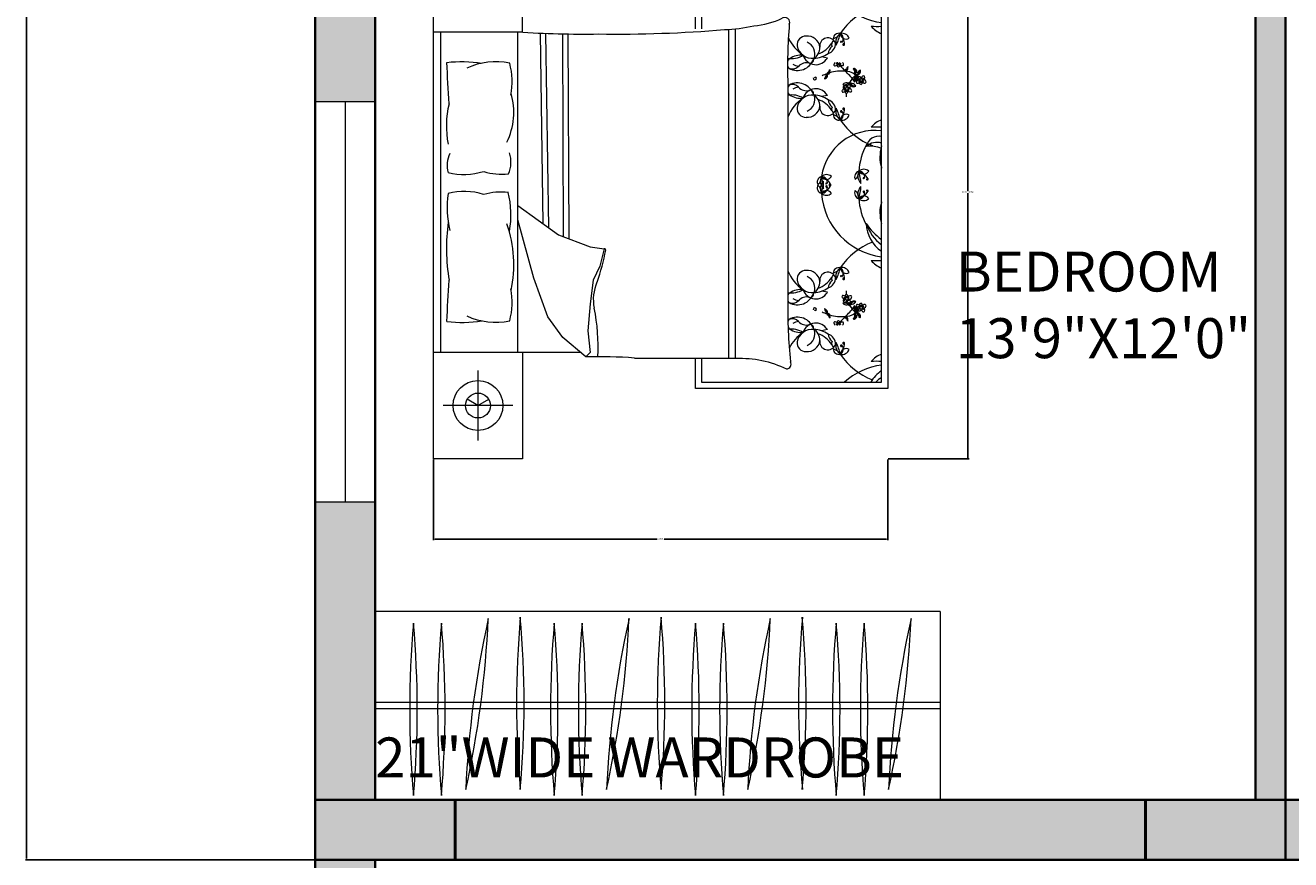
# Model space of a CAD drawing. Units: inches. Extents: x -28 to 485, y -861 to 54.
# Tile 6 of 14: x -28 to 162, y -365 to -240. Entities that reach past the tile are written whole.
import ezdxf

# ---------------------------------------------------------------- set-up
doc = ezdxf.new("R2010")
doc.units = ezdxf.units.IN
doc.header["$MEASUREMENT"] = 0
for name, color, linetype, lineweight in [('A-ANNO-DIMS', 2, 'Continuous', 18), ('A-ANNO-TEXT', 7, 'Continuous', 18), ('A-AREA-IDEN', 7, 'Continuous', 18), ('A-COLS', 7, 'Continuous', 50), ('A-COLS-PATT', 8, 'Continuous', 13), ('A-FLOR-CASE', 8, 'Continuous', 18), ('A-FURN', 8, 'Continuous', 13), ('A-GLAZ', 4, 'Continuous', 18), ('A-WALL', 7, 'Continuous', 35), ('A-WALL-PATT', 34, 'Continuous', 13)]:
    doc.layers.add(name, color=color, linetype=linetype, lineweight=lineweight)
doc.styles.get("Standard").update_dxf_attribs({"font": 'arial.ttf'})
doc.dimstyles.get("Standard").update_dxf_attribs({"dimtxt": 0.18, "dimasz": 0.18, "dimexe": 0.18, "dimexo": 0.0625, "dimgap": 0.09, "dimtad": 0, "dimtih": 1, "dimtoh": 1, "dimdec": 0, "dimzin": 0, "dimdsep": 46, "dimlunit": 3, "dimtxsty": 'Standard', "dimcen": 0.09, "dimadec": 0, "dimazin": 0, "dimtfac": 1, "dimtdec": 0, "dimtofl": 0, "dimtmove": 0, "dimatfit": 3, "dimfxl": 1, "dimtolj": 1, "dimtzin": 0, "dimarcsym": 0})

# ---------------------------------------------------------------- blocks, each defined once
blk = doc.blocks.new('BED-DOUBLE-WITH-NIGHTSTANDS')
for p, q in [((0, 0), (0, 80.08)), ((6.67, 66.84), (6.67, 77.31)), ((11.91, 72.08), (1.44, 72.08)), ((39.26, 64.51), (39.26, 68.96)), ((39.26, 68.96), (68.11, 68.96)), ((68.11, 68.96), (68.11, 10.57)), ((40.19, 68.03), (40.19, 64.5)), ((67.18, 68.03), (40.19, 68.03)), ((67.18, 11.5), (67.18, 68.03)), ((45.25, 64.51), (45.25, 15.09)), ((1.03, 64.07), (1.03, 16.02)), ((12.66, 16.02), (12.66, 64.07)), ((15.98, 63.85), (16.38, 35.34)), ((16.8, 63.82), (17.22, 34.74)), ((19.33, 63.78), (19.45, 33.37)), ((20.15, 63.78), (20.27, 33.06)), ((44.25, 64.43), (44.25, 15.09)), ((59.06, 60.14), (58.15, 60.31)), ((53.12, 56.3), (53.12, 23.78)), ((59.06, 54.54), (58.15, 54.36)), ((12.66, 38.02), (18.76, 33.63)), ((15.04, 27.14), (12.66, 35.87)), ((18.76, 33.63), (23.47, 31.84)), ((23.47, 31.84), (25.57, 31.52)), ((25.57, 31.52), (24.92, 28.93)), ((24.92, 28.93), (23.95, 26.82)), ((17.14, 21.3), (15.04, 27.14)), ((23.95, 26.82), (23.47, 23.25)), ((59.06, 24.99), (58.15, 25.16)), ((23.47, 23.25), (23.14, 19.19)), ((19.41, 18.22), (17.14, 21.3)), ((23.14, 19.19), (23.47, 15.95)), ((59.06, 19.39), (58.15, 19.21)), ((22.82, 15.3), (19.41, 18.22)), ((0, 16.02), (21.98, 16.02)), ((23.47, 15.95), (22.82, 15.3)), ((39.26, 10.57), (39.26, 15.1)), ((40.19, 15.1), (40.19, 11.5)), ((6.67, 13.24), (6.67, 2.78)), ((40.19, 11.5), (67.18, 11.5)), ((68.11, 10.57), (39.26, 10.57)), ((11.91, 8.01), (1.44, 8.01))]:
    blk.add_line(p, q)
for points in [[(0, 64.07), (13.35, 64.07), (13.35, 80.08), (0, 80.08)], [(6.67, 72.08), (5.06, 71.14)], [(6.67, 72.08), (8.29, 71.14)], [(13.35, 16.02), (13.35, 0), (0, 0)], [(6.67, 8.01), (5.06, 8.94)], [(6.67, 8.01), (8.29, 8.94)]]:
    blk.add_lwpolyline(points)
for points in [[(43.62, 64.41, 0.056112), (48.03, 64.99, 0.095341), (52.27, 66.12)], [(2, 59.47, -0.074897), (7.23, 59.37, 0.472817)], [(7.52, 43.09, -0.14099), (2.18, 42.93, -0.235245)], [(7.52, 39.67, 0.14099), (2.18, 39.83, 0.235245)], [(2, 20.62, 0.074897), (7.23, 20.71, -0.472817)], [(30.15, 15.13, 0.001242), (45.35, 15.09, -0.127202), (52.92, 13.49)]]:
    blk.add_lwpolyline(points, format="xyb")
for centre, radius in [((6.67, 72.08), 3.74), ((6.67, 72.08), 1.87), ((64.11, 56.84), 0.204), ((61.96, 55.51), 0.204), ((61.96, 24.02), 0.204), ((64.11, 22.68), 0.204), ((6.67, 8.01), 3.74), ((6.67, 8.01), 1.87)]:
    blk.add_circle(centre, radius)
for centre, radius, start, end in [((69.62, 57.92), 10.46, 111.4092, 145.6135), ((68.59, 75.81), 10.46, 228.1144, 262.255), ((69.99, 70.57), 5.1, 209.8884, 236.5383), ((70.94, 72.4), 6.35, 223.5186, 233.6964), ((52.68, 65.51), 0.73, 336.5219, 123.8264), ((131.01, 58.75), 77.93, 175.2402, 181.8035), ((68.81, 67.71), 4.25, 221.0454, 247.4453), ((66.52, 79.36), 14.47, 266.3481, 272.5919), ((22.44, 207.63), 143.9, 266.1, 270.9282), ((27.68, 251.44), 187.71, 269.1145, 274.8735), ((58.76, 65.61), 6.06, 203.6453, 236.3329), ((55.85, 62.08), 1.35, 88.9462, 185.5144), ((56.04, 61.53), 1.91, 7.1143, 95.0551), ((59.12, 61.97), 1.2, 19.1312, 189.736), ((60.43, 62.21), 0.737, 126.7319, 206.0245), ((60.79, 62.99), 0.867, 76.272, 177.0484), ((59.47, 64.76), 1.79, 284.7031, 328.6173), ((61.96, 62.49), 1.65, 125.7657, 194.5347), ((53.85, 65.41), 7.32, 332.8176, 347.4827), ((61.24, 62.69), 1.16, 20.9613, 102.2885), ((61.86, 63.85), 0.873, 181.7131, 301.5367), ((59, 62.09), 2.64, 2.0648, 41.1598), ((60.59, 63.07), 0.856, 316.2238, 62.3173), ((61.09, 62.57), 0.0682, 20.2667, 316.2271), ((56.85, 62.5), 2.41, 193.079, 274.7067), ((55.32, 60.77), 1.86, 338.5779, 68.4181), ((55.62, 61.86), 2.33, 305.9599, 357.6409), ((56.78, 64.39), 4.3, 273.4924, 303.7117), ((56.48, 64.35), 3.78, 288.2955, 328.7386), ((58.76, 62.26), 1.5, 285.6955, 4.031), ((60.76, 60.64), 1.6, 128.4175, 173.8338), ((61.51, 62.18), 0.13, 168.5166, 2.0648), ((61.45, 62.19), 0.0631, 52.0591, 168.5166), ((-760.15, 15.33), 763.42, 2.85022, 3.31479), ((9.33, 49.26), 10.32, 78.2417, 114.8684), ((1.06, 56.61), 10.73, 348.9631, 14.8961), ((54, 59.28), 0.964, 127.675, 162.5814), ((54, 59.28), 0.964, 196.6343, 225.5483), ((53.71, 63.39), 3.32, 259.249, 301.1782), ((54.57, 60.82), 2.55, 240.8249, 340.7178), ((53.81, 59.69), 1.2, 246.1646, 318.4347), ((55.15, 57.49), 3.09, 85.2696, 124.215), ((55.03, 61.2), 2.3, 240.0851, 262.564), ((55.94, 57.8), 1.64, 74.8529, 138.4347), ((57.33, 61.13), 1.99, 196.8663, 330.0915), ((56.5, 59.87), 0.497, 254.8529, 12.6959), ((55.15, 57.49), 3.09, 53.6555, 57.2989), ((60.19, 59.12), 0.158, 125.0752, 284.7644), ((60.43, 59.18), 0.34, 127.3642, 168.4363), ((60.17, 59.45), 0.49, 277.4968, 341.2737), ((60.56, 59.22), 0.195, 88.1325, 178.8919), ((60.95, 59.02), 0.422, 136.3462, 189.6513), ((60.71, 58.98), 0.176, 189.6513, 312.3208), ((60.75, 59.46), 0.204, 183.2768, 356.7232), ((61.39, 59.1), 0.668, 164.2829, 186.9148), ((60.6, 59.09), 0.334, 312.3208, 40.2111), ((61.31, 59.47), 0.474, 201.6382, 274.947), ((60.68, 58.82), 0.619, 42.3896, 66.5724), ((66.93, 63.72), 7.6, 217.9541, 226.8459), ((61.13, 59.18), 0.337, 10.9597, 52.2379), ((61.33, 59.15), 0.156, 274.947, 37.5263), ((62.33, 58.47), 0.42, 115.5379, 168.6744), ((60.9, 59.07), 1.27, 329.344, 349.7412), ((59.89, 58.78), 2.26, 352.8698, 1.6736), ((57.16, 57.12), 0.251, 169.5864, 349.5616), ((57.25, 57.11), 0.154, 349.5616, 167.2949), ((61.28, 51.56), 6.63, 110.1059, 116.9968), ((59.06, 57.02), 0.42, 129.5056, 182.6421), ((57.85, 58), 1.27, 308.4388, 328.836), ((57.63, 59.02), 2.26, 296.5064, 305.3102), ((57.61, 57.86), 1.29, 336.3901, 344.4871), ((59.01, 57.53), 0.163, 83.9457, 185.6216), ((58.36, 57.69), 0.671, 328.836, 0.8141), ((58.71, 57.49), 0.384, 306.5232, 32.4668), ((59.16, 57.79), 0.163, 112.5583, 214.2343), ((59.06, 58.08), 0.384, 265.7131, 351.6568), ((58.72, 58.29), 0.671, 297.3659, 329.344), ((58.21, 58.87), 1.29, 313.6929, 321.7899), ((59.64, 57.99), 0.42, 115.5379, 168.6744), ((58.21, 58.6), 1.27, 329.344, 349.7412), ((61.28, 51.56), 6.63, 86.1723, 106.4158), ((57.2, 58.31), 2.26, 352.8698, 1.6736), ((61.86, 58.27), 0.163, 112.5583, 214.2343), ((61.75, 58.56), 0.384, 265.7131, 351.6568), ((61.42, 58.77), 0.671, 297.3659, 329.344), ((61.45, 54.86), 3.33, 60.7959, 85.244), ((54.37, 50.07), 10.94, 37.8256, 47.7588), ((60.91, 59.35), 1.29, 313.6929, 321.7899), ((65.87, 54.52), 3.99, 130.182, 149.456), ((63.07, 58.33), 0.228, 33.0979, 123.1364), ((58.05, 55.12), 5.96, 31.1156, 34.8118), ((62.74, 57.94), 0.617, 2.3172, 70.5201), ((63.67, 56.79), 0.658, 139.3812, 199.9959), ((62.44, 57.27), 0.93, 310.9365, 22.7695), ((63.25, 57.78), 0.178, 135.7354, 318.1297), ((62.95, 58.07), 0.236, 315.7354, 31.1156), ((62.75, 57.57), 0.547, 319.3812, 5.5456), ((63.38, 57.79), 0.178, 68.2452, 250.6395), ((62.97, 58), 0.531, 352.6008, 57.1845), ((64.87, 54.44), 3.55, 111.7087, 116.2181), ((61.45, 54.86), 3.33, 47.5083, 55.9967), ((63.48, 58.12), 0.531, 252.8042, 349.6943), ((62.97, 57.17), 0.565, 331.1838, 51.6792), ((63.53, 58.17), 0.236, 248.2452, 323.6254), ((63.33, 58.31), 0.617, 291.7087, 3.0299), ((63.75, 57.1), 0.2, 138.2946, 276.2474), ((63.83, 57.07), 0.278, 358.5719, 143.8954), ((58.93, 61.56), 5.96, 323.6254, 327.3216), ((63.99, 57.29), 0.281, 208.8493, 269.9355), ((63.75, 57.22), 0.321, 274.2123, 318.1587), ((63.81, 58.16), 0.228, 325.6077, 55.6462), ((64.73, 56.9), 0.643, 121.9501, 165.2442), ((64.28, 57.14), 0.135, 262.868, 7.094), ((64.27, 57.26), 0.403, 278.5614, 22.5914), ((64.49, 57.27), 0.202, 44.3732, 121.9501), ((54, 55.39), 0.964, 134.4517, 156.7144), ((54.57, 53.85), 2.55, 19.2822, 119.1751), ((53.81, 54.99), 1.2, 41.5653, 113.8354), ((55.03, 53.47), 2.3, 97.436, 119.9149), ((55.94, 56.87), 1.64, 221.5653, 285.1471), ((57.33, 53.55), 1.99, 29.9085, 163.1337), ((56.5, 54.81), 0.497, 347.3041, 105.1471), ((61.4, 55.17), 0.158, 125.0752, 284.7644), ((61.65, 55.23), 0.34, 93.635, 168.4363), ((61.66, 57.07), 0.93, 253.6301, 325.4631), ((61.92, 55.78), 0.658, 82.0748, 142.6895), ((61.85, 56.68), 0.675, 228.342, 274.9894), ((61.6, 55.76), 0.2, 138.2946, 276.2474), ((61.38, 55.5), 0.49, 277.4968, 341.2737), ((61.68, 55.73), 0.278, 358.5719, 143.8954), ((61.77, 55.27), 0.195, 88.1325, 178.8919), ((61.84, 55.95), 0.281, 208.8493, 269.9355), ((61.6, 55.89), 0.321, 274.2123, 318.1587), ((62.16, 55.06), 0.422, 136.3462, 189.6513), ((61.87, 56.57), 0.565, 273.8774, 357.1501), ((62.6, 55.14), 0.668, 164.2829, 186.9148), ((62.58, 55.56), 0.643, 121.9501, 165.2442), ((62.09, 56.97), 0.547, 262.0748, 308.2393), ((61.81, 55.14), 0.334, 312.3208, 40.2111), ((62.52, 55.52), 0.474, 201.6382, 274.947), ((62.13, 55.81), 0.135, 262.868, 7.094), ((61.89, 54.87), 0.619, 42.3896, 66.5724), ((62.12, 55.92), 0.403, 278.5614, 22.5914), ((62.34, 55.23), 0.337, 10.9597, 118.7804), ((65.87, 54.52), 3.99, 156.1523, 156.9499), ((62.34, 55.94), 0.202, 44.3732, 121.9501), ((62.97, 56.41), 0.565, 181.4625, 249.4747), ((62.87, 56.86), 0.547, 215.1128, 261.2773), ((63.31, 56.83), 0.93, 197.889, 269.722), ((62.55, 55.2), 0.156, 274.947, 37.5263), ((63.02, 56.51), 0.675, 248.3627, 295.0101), ((62.69, 55.67), 0.658, 20.6625, 81.2773), ((62.87, 57.22), 0.675, 285.6484, 332.2957), ((63.55, 56.5), 0.158, 125.0752, 284.7644), ((63.8, 56.56), 0.34, 93.635, 168.4363), ((63.53, 56.83), 0.49, 277.4968, 341.2737), ((63.92, 56.61), 0.195, 88.1325, 178.8919), ((64.31, 56.4), 0.422, 136.3462, 189.6513), ((64.07, 56.36), 0.176, 189.6513, 312.3208), ((64.75, 56.48), 0.668, 164.2829, 186.9148), ((63.96, 56.47), 0.334, 312.3208, 40.2111), ((64.67, 56.85), 0.474, 201.6382, 274.947), ((64.04, 56.2), 0.619, 42.3896, 66.5724), ((64.49, 56.56), 0.337, 10.9597, 118.7804), ((64.7, 56.53), 0.156, 274.947, 37.5263), ((16.01, 49.96), 14.08, 166.3427, 191.1841), ((1.85, 51.98), 10.19, 333.8761, 16.1746), ((54, 55.39), 0.964, 203.2856, 232.325), ((53.71, 51.28), 3.32, 58.8218, 100.2867), ((58.76, 49.06), 6.06, 123.6671, 158.5059), ((55.15, 57.18), 3.09, 235.785, 274.7304), ((56.85, 52.18), 2.41, 85.2933, 166.921), ((55.32, 53.9), 1.86, 291.5819, 21.4221), ((55.15, 57.18), 3.09, 302.7011, 306.3445), ((55.62, 52.81), 2.33, 2.3591, 54.0401), ((56.78, 50.29), 4.3, 56.2883, 86.5076), ((56.48, 50.32), 3.78, 31.2614, 71.7045), ((60.76, 54.03), 1.6, 186.1662, 231.5825), ((58.76, 52.42), 1.5, 355.969, 74.3045), ((61.92, 55.02), 0.176, 189.6513, 312.3208), ((65.87, 54.52), 3.99, 175.2415, 182.8929), ((55.85, 52.59), 1.35, 174.4856, 271.0538), ((56.04, 53.15), 1.91, 264.9449, 352.8857), ((59.12, 52.71), 1.2, 170.264, 340.8688), ((60.43, 52.46), 0.737, 153.9755, 233.2681), ((60.79, 51.69), 0.867, 182.9516, 283.728), ((59.47, 49.92), 1.79, 31.3827, 75.2969), ((61.96, 52.19), 1.65, 165.4653, 234.2343), ((53.85, 49.26), 7.32, 12.5173, 27.1824), ((59, 52.59), 2.64, 318.8402, 357.9352), ((60.59, 51.6), 0.856, 297.6827, 43.7762), ((61.86, 50.82), 0.873, 58.4633, 178.2869), ((61.24, 51.98), 1.16, 257.7115, 339.0387), ((61.13, 52.12), 0.113, 43.7762, 339.7183), ((61.51, 52.5), 0.13, 357.9352, 191.4834), ((61.45, 52.48), 0.0631, 191.4834, 307.9409), ((69.62, 56.75), 10.46, 214.3865, 248.5908), ((68.81, 46.96), 4.25, 112.5547, 138.9546), ((66.52, 35.31), 14.47, 87.4081, 93.6519), ((66.17, 41.19), 8.09, 82.8636, 171.8197), ((66.74, 46.53), 1.88, 76.3898, 169.0739), ((66.48, 45.12), 2.37, 72.8609, 131.9049), ((5.99, 44.03), 3.96, 153.3437, 196.1026), ((7.37, 44.56), 4.25, 335.0183, 18.5407), ((74.19, 42.33), 10.46, 152.5854, 175.5377), ((65.43, 42.24), 4.68, 68.117, 96.6195), ((72.68, 45.26), 5.75, 162.9798, 196.4569), ((75.64, 42.98), 8.5, 174.3643, 175.6213), ((81.47, 38.5), 15.2, 160.0972, 160.2783), ((10.2, 52.53), 9.81, 254.1707, 275.9871), ((58.4, 41.51), 0.867, 106.1963, 206.9726), ((56.38, 42.39), 1.79, 314.6273, 358.5415), ((59.67, 41.66), 1.65, 155.6899, 224.4589), ((58.94, 41.49), 1.16, 50.8855, 132.2127), ((58.91, 42.8), 0.873, 211.6373, 331.4609), ((58.2, 41.49), 0.856, 346.148, 92.2415), ((57.3, 39.84), 2.64, 31.989, 71.0841), ((51.18, 40.16), 7.32, 2.7418, 17.407), ((64.01, 42.31), 0.867, 106.1963, 206.9726), ((61.98, 43.19), 1.79, 314.6273, 358.5415), ((65.27, 42.46), 1.65, 155.6899, 224.4589), ((64.54, 42.29), 1.16, 50.8855, 132.2127), ((64.51, 43.6), 0.873, 211.6373, 331.4609), ((63.8, 42.29), 0.856, 346.148, 92.2415), ((62.91, 40.64), 2.64, 31.989, 71.0841), ((56.78, 40.96), 7.32, 2.7418, 17.407), ((64.47, 42.1), 0.0682, 50.1909, 346.0209), ((64.98, 41.95), 0.0631, 81.9833, 198.4408), ((65.04, 41.98), 0.13, 198.4408, 31.989), ((10.2, 30.23), 9.81, 84.0129, 105.8293), ((-2.51, 36.66), 14.12, 349.8617, 13.6238), ((58.4, 40.68), 0.867, 153.0274, 253.8037), ((56.38, 39.81), 1.79, 1.4585, 45.3727), ((59.67, 40.53), 1.65, 135.5411, 204.3101), ((51.18, 42.04), 7.32, 342.593, 357.2582), ((57.3, 42.35), 2.64, 288.9159, 328.011), ((58.2, 40.71), 0.856, 267.7585, 13.852), ((58.91, 39.39), 0.873, 28.5391, 148.3627), ((58.94, 40.71), 1.16, 227.7873, 309.1145), ((68.59, 40.66), 10.46, 184.4623, 262.255), ((58.87, 41.3), 0.0682, 50.1909, 346.0209), ((58.92, 40.88), 0.113, 13.852, 309.9245), ((59.44, 41.17), 0.13, 198.4408, 31.989), ((59.37, 41.15), 0.0631, 81.9833, 198.4408), ((59.44, 41.02), 0.13, 328.011, 161.5592), ((59.37, 41.04), 0.0631, 161.5592, 278.0167), ((64.01, 39.88), 0.867, 153.0274, 253.8037), ((61.98, 39.01), 1.79, 1.4585, 45.3727), ((65.27, 39.73), 1.65, 135.5411, 204.3101), ((56.78, 41.24), 7.32, 342.593, 357.2582), ((62.91, 41.55), 2.64, 288.9159, 328.011), ((63.8, 39.91), 0.856, 267.7585, 13.852), ((64.52, 40.08), 0.113, 13.852, 309.9245), ((64.98, 40.24), 0.0631, 161.5592, 278.0167), ((65.04, 40.22), 0.13, 328.011, 161.5592), ((16.3, 37.72), 14.27, 171.5249, 193.96), ((64.51, 38.59), 0.873, 28.5391, 148.3627), ((64.54, 39.91), 1.16, 227.7873, 309.1145), ((74.19, 39.86), 10.46, 184.4623, 207.4146), ((72.68, 36.94), 5.75, 163.5431, 197.0202), ((75.64, 39.22), 8.5, 184.3787, 185.6357), ((81.47, 43.7), 15.2, 199.7217, 199.9028), ((30.98, 31.59), 29.04, 172.2196, 189.497), ((-6.57, 29.12), 18.61, 348.0397, 19.2615), ((69.99, 35.42), 5.1, 181.272, 236.5383), ((72.72, 40.59), 9.45, 214.0123, 234.053), ((70.94, 37.25), 6.35, 197.8504, 233.6964), ((69.62, 22.77), 10.46, 111.4092, 145.6135), ((-4.69, 37.08), 31.06, 340.1194, 349.3383), ((25.64, 31.34), 0.193, 358.8623, 109.7536), ((60.79, 27.84), 0.867, 76.272, 177.0484), ((59.47, 29.61), 1.79, 284.7031, 328.6173), ((61.96, 27.34), 1.65, 125.7657, 194.5347), ((53.85, 30.27), 7.32, 332.8176, 347.4827), ((61.24, 27.55), 1.16, 20.9613, 102.2885), ((60.59, 27.92), 0.856, 316.2238, 62.3173), ((59, 26.94), 2.64, 2.0648, 41.1598), ((61.86, 28.71), 0.873, 181.7131, 301.5367), ((66.52, 44.21), 14.47, 266.3481, 272.5919), ((68.81, 32.56), 4.25, 221.0454, 247.4453), ((-760.15, 64.76), 763.42, 356.68521, 357.14978), ((58.76, 30.46), 6.06, 201.4941, 236.3329), ((55.85, 26.93), 1.35, 88.9462, 185.5144), ((56.85, 27.35), 2.41, 193.079, 274.7067), ((56.04, 26.38), 1.91, 7.1143, 95.0551), ((55.32, 25.63), 1.86, 338.5779, 68.4181), ((55.62, 26.71), 2.33, 305.9599, 357.6409), ((56.48, 29.2), 3.78, 288.2955, 328.7386), ((59.12, 26.82), 1.2, 19.1312, 189.736), ((58.76, 27.11), 1.5, 285.6955, 4.031), ((60.76, 25.49), 1.6, 128.4175, 173.8338), ((60.43, 27.07), 0.737, 126.7319, 206.0245), ((61.09, 27.42), 0.0682, 20.2667, 316.2271), ((61.51, 27.03), 0.13, 168.5166, 2.0648), ((61.45, 27.04), 0.0631, 52.0591, 168.5166), ((1.06, 23.47), 10.73, 345.1039, 11.0369), ((30.48, 23.89), 6.52, 156.2616, 191.3392), ((53.71, 28.24), 3.32, 259.7133, 301.1782), ((54, 24.13), 0.964, 127.675, 156.7144), ((54.57, 25.67), 2.55, 240.8249, 340.7178), ((55.15, 22.34), 3.09, 85.2696, 124.215), ((57.33, 25.98), 1.99, 196.8663, 330.0915), ((56.5, 24.72), 0.497, 254.8529, 12.6959), ((55.15, 22.34), 3.09, 53.6555, 57.2989), ((56.78, 29.24), 4.3, 273.4924, 303.7117), ((61.92, 24.5), 0.176, 47.6792, 170.3487), ((65.87, 25.01), 3.99, 177.1071, 184.7585), ((136.48, 22.83), 83.37, 179.3433, 185.6887), ((54, 24.13), 0.964, 203.229, 225.5483), ((53.81, 24.54), 1.2, 246.1646, 318.4347), ((55.03, 26.06), 2.3, 240.0851, 262.564), ((55.94, 22.65), 1.64, 74.8529, 138.4347), ((61.4, 24.36), 0.158, 75.2356, 234.9248), ((61.65, 24.3), 0.34, 191.5637, 266.365), ((61.6, 23.76), 0.2, 83.7526, 221.7054), ((61.85, 22.84), 0.675, 85.0106, 131.658), ((61.66, 22.46), 0.93, 34.5369, 106.3699), ((61.92, 23.75), 0.658, 217.3105, 277.9252), ((61.38, 24.03), 0.49, 18.7263, 82.5032), ((61.68, 23.79), 0.278, 216.1046, 1.4281), ((61.77, 24.25), 0.195, 181.1081, 271.8675), ((61.84, 23.57), 0.281, 90.0645, 151.1507), ((61.6, 23.64), 0.321, 41.8413, 85.7877), ((62.16, 24.46), 0.422, 170.3487, 223.6538), ((61.87, 22.95), 0.565, 2.8499, 86.1226), ((62.6, 24.38), 0.668, 173.0852, 195.7171), ((62.58, 23.96), 0.643, 194.7558, 238.0499), ((62.09, 22.55), 0.547, 51.7607, 97.9252), ((61.81, 24.39), 0.334, 319.7889, 47.6792), ((62.52, 24.01), 0.474, 85.053, 158.3618), ((62.13, 23.71), 0.135, 352.906, 97.132), ((61.89, 24.66), 0.619, 293.4276, 317.6104), ((62.34, 24.29), 0.337, 241.2196, 349.0403), ((62.12, 23.6), 0.403, 337.4086, 81.4386), ((65.87, 25.01), 3.99, 203.0501, 203.8477), ((62.34, 23.59), 0.202, 238.0499, 315.6268), ((62.97, 23.11), 0.565, 110.5253, 178.5375), ((63.31, 22.7), 0.93, 90.278, 162.111), ((62.87, 22.67), 0.547, 98.7227, 144.8872), ((65.87, 25.01), 3.99, 210.544, 229.818), ((62.55, 24.33), 0.156, 322.4737, 85.053), ((63.02, 23.01), 0.675, 64.9899, 111.6373), ((62.69, 23.86), 0.658, 278.7227, 339.3375), ((63.67, 22.74), 0.658, 160.0041, 220.6188), ((62.44, 22.26), 0.93, 337.2305, 49.0635), ((62.87, 22.31), 0.675, 27.7043, 74.3516), ((63.55, 23.03), 0.158, 75.2356, 234.9248), ((63.8, 22.96), 0.34, 191.5637, 266.365), ((63.53, 22.69), 0.49, 18.7263, 82.5032), ((63.92, 22.92), 0.195, 181.1081, 271.8675), ((64.07, 23.17), 0.176, 47.6792, 170.3487), ((64.31, 23.13), 0.422, 170.3487, 223.6538), ((64.75, 23.05), 0.668, 173.0852, 195.7171), ((63.96, 23.05), 0.334, 319.7889, 47.6792), ((64.67, 22.68), 0.474, 85.053, 158.3618), ((64.04, 23.32), 0.619, 293.4276, 317.6104), ((64.49, 22.96), 0.337, 241.2196, 349.0403), ((64.7, 22.99), 0.156, 322.4737, 85.053), ((9.33, 30.82), 10.32, 245.1316, 281.7583), ((-5.54, 16.67), 30.23, 357.4519, 11.3392), ((54, 20.25), 0.964, 134.4517, 153.558), ((54.57, 18.71), 2.55, 19.2822, 119.1751), ((53.81, 19.84), 1.2, 41.5653, 113.8354), ((57.16, 22.4), 0.251, 10.4384, 190.4136), ((57.25, 22.42), 0.154, 192.7051, 10.4384), ((61.28, 27.97), 6.63, 243.0032, 249.8941), ((57.85, 21.53), 1.27, 31.164, 51.5612), ((59.06, 22.5), 0.42, 177.3579, 230.4944), ((57.63, 20.5), 2.26, 54.6898, 63.4936), ((57.61, 21.66), 1.29, 15.5129, 23.6099), ((59.01, 21.99), 0.163, 174.3784, 276.0543), ((58.71, 22.03), 0.384, 327.5332, 53.4768), ((58.36, 21.84), 0.671, 359.1859, 31.164), ((59.16, 21.74), 0.163, 145.7657, 247.4417), ((59.06, 21.45), 0.384, 8.3432, 94.2869), ((58.72, 21.23), 0.671, 30.656, 62.6341), ((58.21, 20.66), 1.29, 38.2101, 46.3071), ((59.64, 21.53), 0.42, 191.3256, 244.4621), ((58.21, 20.93), 1.27, 10.2588, 30.656), ((61.28, 27.97), 6.63, 253.5842, 273.8277), ((57.2, 21.22), 2.26, 358.3264, 7.1302), ((66.93, 15.8), 7.6, 133.1541, 142.0459), ((61.86, 21.26), 0.163, 145.7657, 247.4417), ((54.37, 29.45), 10.94, 312.2412, 322.1744), ((61.45, 24.67), 3.33, 274.756, 299.2041), ((61.75, 20.97), 0.384, 8.3432, 94.2869), ((61.42, 20.76), 0.671, 30.656, 62.6341), ((60.91, 20.18), 1.29, 38.2101, 46.3071), ((62.33, 21.06), 0.42, 191.3256, 244.4621), ((60.9, 20.45), 1.27, 10.2588, 30.656), ((59.89, 20.74), 2.26, 358.3264, 7.1302), ((62.74, 21.59), 0.617, 289.4799, 357.6828), ((58.05, 24.41), 5.96, 325.1882, 328.8844), ((63.07, 21.2), 0.228, 236.8636, 326.9021), ((63.25, 21.74), 0.178, 41.8703, 224.2646), ((62.95, 21.45), 0.236, 328.8844, 44.2646), ((62.75, 21.95), 0.547, 354.4544, 40.6188), ((63.38, 21.74), 0.178, 109.3605, 291.7548), ((62.97, 21.52), 0.531, 302.8155, 7.3992), ((64.87, 25.09), 3.55, 243.7819, 248.2913), ((61.45, 24.67), 3.33, 304.0033, 312.4917), ((62.97, 22.35), 0.565, 308.3208, 28.8162), ((63.48, 21.4), 0.531, 10.3057, 107.1958), ((63.53, 21.36), 0.236, 36.3746, 111.7548), ((63.75, 22.43), 0.2, 83.7526, 221.7054), ((63.33, 21.21), 0.617, 356.9701, 68.2913), ((63.83, 22.46), 0.278, 216.1046, 1.4281), ((58.93, 17.96), 5.96, 32.6784, 36.3746), ((63.99, 22.24), 0.281, 90.0645, 151.1507), ((63.75, 22.31), 0.321, 41.8413, 85.7877), ((63.81, 21.37), 0.228, 304.3538, 34.3923), ((64.73, 22.63), 0.643, 194.7558, 238.0499), ((64.28, 22.38), 0.135, 352.906, 97.132), ((64.27, 22.27), 0.403, 337.4086, 81.4386), ((64.49, 22.25), 0.202, 238.0499, 315.6268), ((54, 20.25), 0.964, 210.0293, 232.325), ((53.71, 16.14), 3.32, 58.8218, 99.1554), ((55.15, 22.04), 3.09, 235.785, 274.7304), ((55.03, 18.32), 2.3, 97.436, 119.9149), ((56.85, 17.03), 2.41, 85.2933, 166.921), ((55.94, 21.72), 1.64, 221.5653, 285.1471), ((57.33, 18.4), 1.99, 29.9085, 163.1337), ((55.32, 18.75), 1.86, 291.5819, 21.4221), ((56.5, 19.66), 0.497, 347.3041, 105.1471), ((55.15, 22.04), 3.09, 302.7011, 306.3445), ((55.62, 17.67), 2.33, 2.3591, 54.0401), ((56.78, 15.14), 4.3, 56.2883, 86.5076), ((60.19, 20.41), 0.158, 75.2356, 234.9248), ((60.43, 20.35), 0.34, 191.5637, 232.6358), ((60.17, 20.07), 0.49, 18.7263, 82.5032), ((60.56, 20.3), 0.195, 181.1081, 271.8675), ((60.71, 20.55), 0.176, 47.6792, 170.3487), ((60.95, 20.51), 0.422, 170.3487, 223.6538), ((60.75, 20.06), 0.204, 3.2768, 176.7232), ((61.39, 20.43), 0.668, 173.0852, 195.7171), ((60.6, 20.43), 0.334, 319.7889, 47.6792), ((61.31, 20.06), 0.474, 85.053, 158.3618), ((60.68, 20.7), 0.619, 293.4276, 317.6104), ((61.13, 20.34), 0.337, 307.7621, 349.0403), ((61.33, 20.37), 0.156, 322.4737, 85.053), ((58.76, 13.91), 6.06, 123.6671, 153.2997), ((55.85, 17.44), 1.35, 174.4856, 271.0538), ((56.04, 18), 1.91, 264.9449, 352.8857), ((56.48, 15.18), 3.78, 31.2614, 71.7045), ((59.12, 17.56), 1.2, 170.264, 340.8688), ((58.76, 17.27), 1.5, 355.969, 74.3045), ((60.76, 18.89), 1.6, 186.1662, 231.5825), ((60.43, 17.31), 0.737, 153.9755, 233.2681), ((61.96, 17.04), 1.65, 165.4653, 234.2343), ((53.85, 14.11), 7.32, 12.5173, 27.1824), ((59, 17.44), 2.64, 318.8402, 357.9352), ((61.13, 16.97), 0.113, 43.7762, 339.7183), ((61.51, 17.35), 0.13, 357.9352, 191.4834), ((61.45, 17.33), 0.0631, 191.4834, 307.9409), ((24.81, -58.13), 73.46, 85.8294, 91.553), ((59.47, 14.77), 1.79, 31.3827, 75.2969), ((60.79, 16.54), 0.867, 182.9516, 283.728), ((60.59, 16.46), 0.856, 297.6827, 43.7762), ((61.86, 15.67), 0.873, 58.4633, 178.2869), ((61.24, 16.83), 1.16, 257.7115, 339.0387), ((69.62, 21.6), 10.46, 214.3865, 248.5908), ((68.81, 11.81), 4.25, 112.5547, 138.9546), ((52.87, 14.23), 0.739, 273.98, 27.3412), ((68.59, 3.71), 10.46, 97.745, 131.8856), ((66.52, 0.17), 14.47, 87.4081, 93.6519), ((69.99, 8.96), 5.1, 123.4617, 150.1116), ((70.94, 7.13), 6.35, 126.3036, 136.4814)]:
    blk.add_arc(centre, radius, start, end)
blk = doc.blocks.new('WARDROBE-HANGING')
for p, q in [((84.7, 28.23), (0, 28.23)), ((0, 28.23), (0, 0)), ((84.7, 28.23), (84.7, 0)), ((84.7, 14.59), (0, 14.59)), ((84.7, 13.65), (0, 13.65)), ((84.7, 0), (0, 0))]:
    blk.add_line(p, q)
for centre, start, end in [((-131.46, 33.65), 347.508, 357.5023), ((162.01, -4.96), 167.508, 177.5023), ((169.76, 14.46), 175.0028, 184.9972), ((-126.23, 14.46), 355.0028, 4.9972), ((-110.36, 33.65), 347.508, 357.5023), ((183.11, -4.96), 167.508, 177.5023), ((190.86, 14.46), 175.0028, 184.9972), ((-105.13, 14.46), 355.0028, 4.9972), ((204.29, -4.96), 167.508, 177.5023), ((-89.17, 33.65), 347.508, 357.5023), ((212.05, 14.46), 175.0028, 184.9972), ((-83.95, 14.46), 355.0028, 4.9972), ((225.4, -4.96), 167.508, 177.5023), ((-68.07, 33.65), 347.508, 357.5023), ((153.74, 13.55), 175.0028, 184.9972), ((-142.25, 13.55), 355.0028, 4.9972), ((157.93, 13.55), 175.0028, 184.9972), ((-138.07, 13.55), 355.0028, 4.9972), ((174.85, 13.55), 175.0028, 184.9972), ((-121.15, 13.55), 355.0028, 4.9972), ((179.03, 13.55), 175.0028, 184.9972), ((-116.97, 13.55), 355.0028, 4.9972), ((196.03, 13.55), 175.0028, 184.9972), ((-99.97, 13.55), 355.0028, 4.9972), ((200.21, 13.55), 175.0028, 184.9972), ((-95.78, 13.55), 355.0028, 4.9972), ((217.13, 13.55), 175.0028, 184.9972), ((-78.86, 13.55), 355.0028, 4.9972), ((221.31, 13.55), 175.0028, 184.9972), ((-74.68, 13.55), 355.0028, 4.9972)]:
    blk.add_arc(centre, 148.56, start, end)
blk = doc.blocks.new('WINDOW-60IN')
for p, q in [((0, 60), (0, 0)), ((9, 60), (0, 60)), ((4.5, 60), (4.5, 0)), ((9, 0), (9, 60)), ((0, 0), (9, 0))]:
    blk.add_line(p, q)
blk = doc.blocks.new('*D24')
at = {"layer": 'A-ANNO-DIMS', "color": 0, "lineweight": -2, "transparency": 16777216}
for p, q in [((101.2, -224.66), (113.33, -224.66)), ((113.15, -224.84), (113.15, -264.52)), ((113.15, -304.56), (113.15, -264.88)), ((101.2, -304.74), (113.33, -304.74))]:
    blk.add_line(p, q, dxfattribs=at)
at = {"layer": 'A-ANNO-DIMS', "color": 0, "transparency": 16777216}
for points in [[(113.12, -224.84), (113.18, -224.84), (113.15, -224.66)], [(113.12, -304.56), (113.18, -304.56), (113.15, -304.74)]]:
    blk.add_solid(points, dxfattribs=at)
at = {"layer": 'Defpoints', "color": 0, "transparency": 16777216}
for p in [(101.14, -224.66), (113.15, -224.66), (101.14, -304.74)]:
    blk.add_point(p, dxfattribs=at)
at = {"layer": 'A-ANNO-DIMS', "color": 0, "transparency": 16777216, "insert": (113.15, -264.7), "char_height": 0.18, "attachment_point": 5}
blk.add_mtext('\\A1;BED SET 80 TYP.', dxfattribs=at)
blk = doc.blocks.new('*D25')
at = {"layer": 'A-ANNO-DIMS', "color": 0, "lineweight": -2, "transparency": 16777216}
for p, q in [((33.03, -304.81), (33.03, -316.94)), ((101.14, -304.81), (101.14, -316.94)), ((33.21, -316.76), (66.56, -316.76)), ((100.96, -316.76), (67.61, -316.76))]:
    blk.add_line(p, q, dxfattribs=at)
at = {"layer": 'A-ANNO-DIMS', "color": 0, "transparency": 16777216}
for points in [[(33.21, -316.73), (33.21, -316.79), (33.03, -316.76)], [(100.96, -316.73), (100.96, -316.79), (101.14, -316.76)]]:
    blk.add_solid(points, dxfattribs=at)
at = {"layer": 'Defpoints', "color": 0, "transparency": 16777216}
for p in [(33.03, -304.74), (101.14, -304.74), (101.14, -316.76)]:
    blk.add_point(p, dxfattribs=at)
at = {"layer": 'A-ANNO-DIMS', "color": 0, "transparency": 16777216, "insert": (67.09, -316.76), "char_height": 0.18, "attachment_point": 5}
blk.add_mtext('\\A1;68 TYP.', dxfattribs=at)
blk = doc.blocks.new('*D54')
at = {"layer": 'A-ANNO-DIMS', "color": 0, "lineweight": -2, "transparency": 16777216}
for p, q in [((15.22, 10.13), (-28.15, 10.13)), ((-27.97, 9.95), (-27.97, -177.18)), ((-27.97, -364.69), (-27.97, -177.55)), ((15.22, -364.87), (-28.15, -364.87))]:
    blk.add_line(p, q, dxfattribs=at)
at = {"layer": 'A-ANNO-DIMS', "color": 0, "transparency": 16777216}
for points in [[(-28, 9.95), (-27.94, 9.95), (-27.97, 10.13)], [(-28, -364.69), (-27.94, -364.69), (-27.97, -364.87)]]:
    blk.add_solid(points, dxfattribs=at)
at = {"layer": 'Defpoints', "color": 0, "transparency": 16777216}
for p in [(15.28, 10.13), (-27.97, -364.87), (15.28, -364.87)]:
    blk.add_point(p, dxfattribs=at)
at = {"layer": 'A-ANNO-DIMS', "color": 0, "transparency": 16777216, "insert": (-27.97, -177.37), "char_height": 0.18, "attachment_point": 5}
blk.add_mtext('\\A1;375', dxfattribs=at)

msp = doc.modelspace()

# ---------------------------------------------------------------- hatches: boundary and pattern name
at = {"layer": 'A-COLS-PATT'}
h = msp.add_hatch(color=256, dxfattribs=at)
h.dxf.hatch_style = 1
h.paths.add_polyline_path([(36.285, 10.133), (15.285, 10.133), (15.285, 1.133), (36.285, 1.133)])
h.paths.add_polyline_path([(160.785, 10.133), (139.785, 10.133), (139.785, 1.133), (160.785, 1.133)])
h.paths.add_polyline_path([(316.785, 10.133), (295.785, 10.133), (295.785, 1.133), (316.785, 1.133)])
h.paths.add_polyline_path([(441.285, 10.133), (420.285, 10.133), (420.285, 1.133), (441.285, 1.133)])
h.paths.add_polyline_path([(441.285, -138.367), (432.285, -138.367), (420.285, -138.367), (420.285, -147.367), (441.285, -147.367)])
h.paths.add_polyline_path([(304.785, -130.867), (295.785, -130.867), (295.785, -147.367), (304.785, -147.367), (304.785, -142.867)])
h.paths.add_polyline_path([(160.785, -130.867), (151.785, -130.867), (151.785, -142.867), (151.785, -147.367), (160.785, -147.367)])
h.paths.add_polyline_path([(36.285, -138.367), (24.285, -138.367), (15.285, -138.367), (15.285, -147.367), (36.285, -147.367)])
h.paths.add_polyline_path([(36.285, -355.867), (15.285, -355.867), (15.285, -364.867), (36.285, -364.867)])
h.paths.add_polyline_path([(160.785, -355.867), (139.785, -355.867), (139.785, -364.867), (160.785, -364.867)])
h.paths.add_polyline_path([(316.785, -355.867), (300.285, -355.867), (295.785, -355.867), (295.785, -364.867), (316.785, -364.867)])
at = {"layer": 'A-WALL-PATT'}
h = msp.add_hatch(color=256, dxfattribs=at)
h.dxf.hatch_style = 1
h.paths.add_polyline_path([(160.785, -808.867), (160.785, -817.867), (295.785, -817.867), (295.785, -808.867)])
h.paths.add_polyline_path([(316.785, -817.867), (323.776, -817.867), (323.776, -808.867), (316.785, -808.867)])
h.paths.add_polyline_path([(420.285, -817.867), (420.285, -808.867), (383.776, -808.867), (383.776, -817.867)])
h.paths.add_polyline_path([(432.285, -808.867), (441.285, -808.867), (441.285, -702.966), (432.285, -702.966), (432.285, -708.367), (397.785, -708.367), (397.785, -710.617), (397.785, -712.867), (432.285, -712.867)])
h.paths.add_polyline_path([(300.285, -712.867), (329.285, -712.867), (329.285, -710.617), (329.285, -708.367), (295.785, -708.367), (295.785, -808.867), (300.285, -808.867)])
h.paths.add_polyline_path([(160.785, -698.867), (158.535, -698.867), (156.285, -698.867), (156.285, -808.867), (160.785, -808.867)])
h.paths.add_polyline_path([(36.285, -808.867), (36.285, -817.867), (79.721, -817.867), (79.721, -808.867)])
h.paths.add_polyline_path([(15.285, -808.867), (24.285, -808.867), (24.285, -739.09), (15.285, -739.09)])
h.paths.add_polyline_path([(24.285, -640.781), (15.285, -640.781), (15.285, -679.09), (24.285, -679.09), (24.285, -664.867), (89.285, -664.867), (89.285, -662.617), (89.285, -660.367), (24.285, -660.367)])
h.paths.add_polyline_path([(15.285, -616.781), (24.285, -616.781), (24.285, -600.367), (15.285, -600.367)])
h.paths.add_polyline_path([(36.285, -595.867), (36.285, -600.367), (123.285, -600.367), (123.285, -660.367), (117.285, -660.367), (117.285, -664.867), (156.285, -664.867), (156.285, -670.867), (160.785, -670.867), (160.785, -660.367), (127.785, -660.367), (127.785, -600.367), (129.785, -600.367), (129.785, -598.117), (129.785, -595.867)])
h.paths.add_polyline_path([(367.785, -664.867), (363.285, -664.867), (363.285, -708.367), (357.285, -708.367), (357.285, -712.867), (369.785, -712.867), (369.785, -708.367), (367.785, -708.367)])
h.paths.add_polyline_path([(432.285, -664.867), (432.285, -666.966), (441.285, -666.966), (441.285, -642.367), (432.285, -642.367), (432.285, -660.367), (328.785, -660.367), (328.785, -664.867), (363.285, -664.867)])
h.paths.add_polyline_path([(333.285, -600.367), (420.285, -600.367), (420.285, -595.867), (326.785, -595.867), (326.785, -600.367), (328.785, -600.367), (328.785, -630.367), (331.035, -630.367), (333.285, -630.367)])
h.paths.add_polyline_path([(441.285, -600.367), (432.285, -600.367), (432.285, -618.367), (441.285, -618.367)])
h.paths.add_polyline_path([(432.285, -591.367), (441.285, -591.367), (441.285, -547.793), (432.285, -547.793)])
h.paths.add_polyline_path([(295.785, -588.367), (300.238, -588.367), (300.285, -583.867), (300.285, -451.867), (295.785, -451.867)])
h.paths.add_polyline_path([(420.285, -451.867), (420.285, -442.867), (316.785, -442.867), (316.785, -451.867)])
h.paths.add_polyline_path([(432.285, -487.793), (441.285, -487.793), (441.285, -451.867), (432.285, -451.867)])
h.paths.add_polyline_path([(432.285, -442.867), (441.285, -442.867), (441.285, -364.867), (432.285, -364.867)])
h.paths.add_polyline_path([(261.785, -451.867), (261.785, -447.367), (261.785, -444.758), (261.785, -442.867), (160.785, -442.867), (160.785, -451.867)])
h.paths.add_polyline_path([(139.785, -451.867), (139.785, -442.867), (36.285, -442.867), (36.285, -451.867)])
h.paths.add_polyline_path([(15.285, -491.617), (24.285, -491.617), (24.285, -451.867), (15.285, -451.867)])
h.paths.add_polyline_path([(24.285, -551.617), (15.285, -551.617), (15.285, -591.367), (24.285, -591.367)])
h.paths.add_polyline_path([(160.785, -451.867), (156.285, -451.867), (156.285, -588.367), (160.785, -588.367)])
h.paths.add_polyline_path([(139.785, -364.867), (139.785, -355.867), (36.285, -355.867), (36.285, -364.867)])
h.paths.add_polyline_path([(24.285, -364.867), (15.285, -364.867), (15.285, -373.867), (24.285, -373.867)])
h.paths.add_polyline_path([(15.285, -433.867), (15.285, -442.867), (24.285, -442.867), (24.285, -433.867)])
h.paths.add_polyline_path([(261.785, -364.867), (261.785, -360.367), (261.785, -355.867), (160.785, -355.867), (160.785, -364.867)])
h.paths.add_polyline_path([(295.785, -355.867), (289.785, -355.867), (289.785, -364.867), (295.785, -364.867)])
h.paths.add_polyline_path([(295.785, -355.867), (300.285, -355.867), (300.285, -259.867), (333.285, -259.867), (333.285, -257.617), (333.285, -255.367), (300.285, -255.367), (300.285, -207.367), (295.785, -207.367)])
h.paths.add_polyline_path([(420.285, -364.867), (420.285, -355.867), (316.785, -355.867), (316.785, -364.867)])
h.paths.add_polyline_path([(24.285, -311.192), (15.285, -311.192), (15.285, -355.867), (24.285, -355.867)])
h.paths.add_polyline_path([(24.285, -211.867), (54.144, -211.867), (54.144, -207.367), (24.285, -207.367), (24.285, -187.772), (15.285, -187.772), (15.285, -251.192), (24.285, -251.192)])
h.paths.add_polyline_path([(82.144, -207.367), (82.144, -209.617), (82.144, -211.867), (127.785, -211.867), (127.785, -147.367), (129.785, -147.367), (129.785, -145.117), (129.785, -142.867), (36.285, -142.867), (36.285, -147.367), (123.285, -147.367), (123.285, -207.367)])
h.paths.add_polyline_path([(160.785, -207.367), (156.285, -207.367), (156.285, -355.867), (160.785, -355.867)])
h.paths.add_polyline_path([(24.285, 1.133), (15.285, 1.133), (15.285, -54.408), (24.285, -54.408)])
h.paths.add_polyline_path([(36.285, 10.133), (36.285, 1.133), (70.235, 1.133), (70.235, 10.133)])
h.paths.add_polyline_path([(15.285, -138.367), (24.285, -138.367), (24.285, -114.408), (15.285, -114.408)])
h.paths.add_polyline_path([(24.285, -147.367), (15.285, -147.367), (15.285, -163.772), (24.285, -163.772)])
h.paths.add_polyline_path([(156.285, -130.867), (160.785, -130.867), (160.785, 1.133), (156.285, 1.133)])
h.paths.add_polyline_path([(130.235, 1.133), (139.785, 1.133), (139.785, 10.133), (130.235, 10.133)])
h.paths.add_polyline_path([(316.785, 10.133), (316.785, 1.133), (328.097, 1.133), (328.097, 10.133)])
h.paths.add_polyline_path([(300.285, 1.133), (295.785, 1.133), (295.785, -130.867), (300.285, -130.867)])
h.paths.add_polyline_path([(420.285, -147.367), (420.285, -142.867), (326.785, -142.867), (326.785, -145.117), (326.785, -147.367), (328.785, -147.367), (328.785, -177.367), (331.035, -177.367), (333.285, -177.367), (333.285, -147.367)])
h.paths.add_polyline_path([(333.285, -207.367), (333.285, -205.367), (328.785, -205.367), (328.785, -211.867), (363.285, -211.867), (363.285, -255.367), (361.285, -255.367), (361.285, -259.867), (369.785, -259.867), (369.785, -255.367), (367.785, -255.367), (367.785, -211.867), (432.285, -211.867), (432.285, -214.893), (441.285, -214.893), (441.285, -188.008), (432.285, -188.008), (432.285, -207.367)])
h.paths.add_polyline_path([(441.285, -250.893), (432.285, -250.893), (432.285, -255.367), (397.785, -255.367), (397.785, -257.617), (397.785, -259.867), (432.285, -259.867), (432.285, -355.867), (441.285, -355.867)])
h.paths.add_polyline_path([(432.285, -138.367), (441.285, -138.367), (441.285, -115.099), (432.285, -115.099)])
h.paths.add_polyline_path([(441.285, -147.367), (432.285, -147.367), (432.285, -164.008), (441.285, -164.008)])
h.paths.add_polyline_path([(420.285, 1.133), (420.285, 10.133), (388.097, 10.133), (388.097, 1.133)])
h.paths.add_polyline_path([(432.285, -55.099), (441.285, -55.099), (441.285, 1.133), (432.285, 1.133)])

# ---------------------------------------------------------------- linework, layer by layer
at = {"layer": 'A-COLS'}
for p, q in [((36.285, -355.867), (36.285, -364.867)), ((139.785, -355.867), (139.785, -364.867))]:
    msp.add_line(p, q, dxfattribs=at)
at = {"layer": 'A-WALL'}
for p, q in [((15.285, 10.133), (15.285, -817.867)), ((160.785, 10.133), (160.785, -364.867)), ((156.285, -147.367), (156.285, -355.867)), ((24.285, -211.867), (24.285, -355.867)), ((15.285, -355.867), (261.785, -355.867)), ((15.285, -364.867), (345.285, -364.867)), ((24.285, -364.867), (24.285, -442.867))]:
    msp.add_line(p, q, dxfattribs=at)

# ---------------------------------------------------------------- block references
at = {"layer": 'A-FLOR-CASE'}
msp.add_blockref('WARDROBE-HANGING', (24.285, -355.867), dxfattribs=at)
at = {"layer": 'A-FURN'}
msp.add_blockref('BED-DOUBLE-WITH-NIGHTSTANDS', (33.033, -304.743), dxfattribs=at)
at = {"layer": 'A-GLAZ'}
msp.add_blockref('WINDOW-60IN', (15.285, -311.192), dxfattribs=at)

# ---------------------------------------------------------------- texts
at = {"layer": 'A-ANNO-TEXT', "insert": (24.285, -346.531), "char_height": 6, "attachment_point": 1}
msp.add_mtext('21"WIDE WARDROBE', dxfattribs=at)
at = {"layer": 'A-AREA-IDEN', "insert": (111.355, -273.632), "char_height": 6, "attachment_point": 1}
msp.add_mtext('BEDROOM\\P13\'9"X12\'0"', dxfattribs=at)

# ---------------------------------------------------------------- dimensions: what is measured, and where the dimension line sits
at = {"layer": 'A-ANNO-DIMS'}
dim = msp.add_linear_dim(base=(-27.965, -364.867), p1=(15.285, 10.133), p2=(15.285, -364.867), angle=90, dimstyle='Standard', override={"dimdec": 0, "dimlfac": 1, "dimrnd": 0, "dimzin": 0, "dimdsep": 46, "dimlunit": 2}, dxfattribs=at)
dim.commit()
dim.dimension.update_dxf_attribs({"geometry": '*D54', "text_midpoint": (-27.965, -177.367)})
dim = msp.add_linear_dim(base=(113.152, -224.659), p1=(101.14, -304.743), p2=(101.14, -224.659), angle=90, text='BED SET <> TYP.', dimstyle='Standard', override={"dimdec": 0, "dimlfac": 1, "dimrnd": 0, "dimzin": 0, "dimdsep": 46, "dimlunit": 2}, dxfattribs=at)
dim.commit()
dim.dimension.update_dxf_attribs({"geometry": '*D24', "text_midpoint": (113.152, -264.701)})
dim = msp.add_linear_dim(base=(101.14, -316.756), p1=(33.033, -304.743), p2=(101.14, -304.743), text='<> TYP.', dimstyle='Standard', override={"dimdec": 0, "dimlfac": 1, "dimrnd": 0, "dimzin": 0, "dimdsep": 46, "dimlunit": 2}, dxfattribs=at)
dim.commit()
dim.dimension.update_dxf_attribs({"geometry": '*D25', "text_midpoint": (67.086, -316.756)})

doc.saveas('drawing.dxf')
